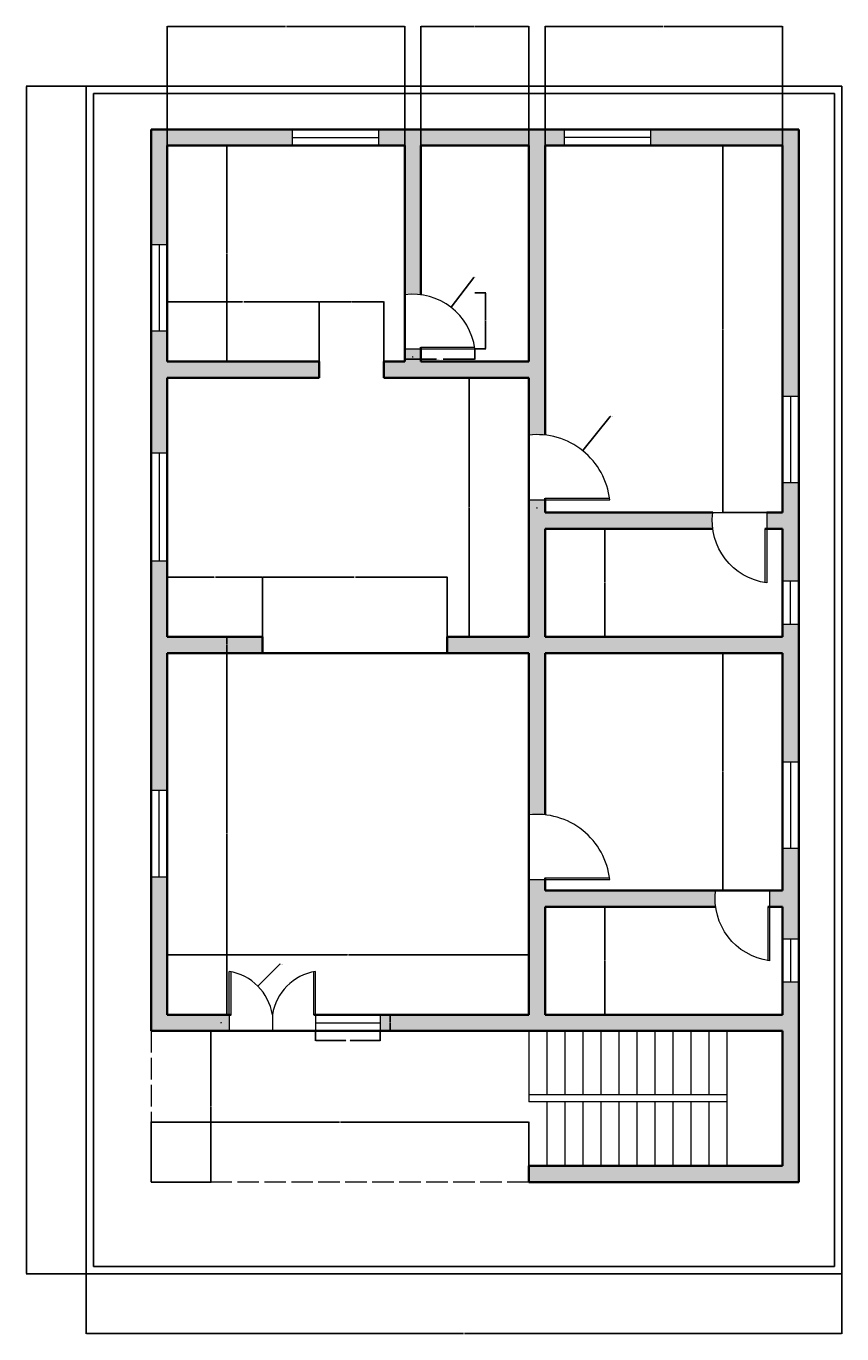
# Model space of a CAD drawing. Units: inches. Extents: x 4948 to 20975, y 6797 to 20508.
# Tile 5 of 5: x 20521 to 20975, y 19252 to 19979. Entities that reach past the tile are written whole.
import ezdxf

# ---------------------------------------------------------------- set-up
doc = ezdxf.new("R2010")
doc.units = ezdxf.units.IN
doc.linetypes.add('ACAD_ISO02W100', pattern=[15, 12, -3])
for name, color, linetype, lineweight in [('A-ANNO-DIMS', 2, 'Continuous', 18), ('A-DOOR', 3, 'Continuous', 18), ('A-FLOR-OVHD', 8, 'ACAD_ISO02W100', 18), ('A-FLOR-STRS', 7, 'Continuous', 18), ('A-GLAZ', 4, 'Continuous', 18), ('A-WALL', 7, 'Continuous', 35), ('C-PROP', 7, 'Continuous', 25)]:
    doc.layers.add(name, color=color, linetype=linetype, lineweight=lineweight)
doc.layers.add('A-WALL-PATT', color=18, linetype='Continuous', lineweight=13, true_color=0x000000)
doc.styles.get("Standard").update_dxf_attribs({"font": 'times.ttf'})
doc.dimstyles.get("Standard").update_dxf_attribs({"dimtxt": 0.18, "dimasz": 0.18, "dimexe": 0.18, "dimexo": 0.0625, "dimgap": 0.09, "dimtad": 0, "dimtih": 1, "dimtoh": 1, "dimdec": 4, "dimzin": 0, "dimdsep": 46, "dimtxsty": 'Standard', "dimcen": 0.09, "dimadec": 0, "dimazin": 0, "dimtfac": 1, "dimtdec": 4, "dimtofl": 0, "dimtmove": 0, "dimatfit": 3, "dimfxl": 1, "dimtolj": 1, "dimtzin": 0, "dimarcsym": 0})

# ---------------------------------------------------------------- blocks, each defined once
blk = doc.blocks.new('DOOR-SINGLE-36IN')
for p, q in [((9, 1), (45, 1)), ((0, 0), (9, 0)), ((9, 0), (45, 0))]:
    blk.add_line(p, q)
blk.add_arc((4.5, -4.5), 40.75, 6.34019, 96.34019)
blk = doc.blocks.new('DOOR-SINGLE-30IN')
for p, q in [((0, 0), (9, 0)), ((9, 1), (39, 1)), ((9, 0), (39, 0))]:
    blk.add_line(p, q)
blk.add_arc((4.5, -4.5), 34.79, 7.43141, 97.43141)
blk = doc.blocks.new('DOOR-DOUBLE-48IN')
for p, q in [((0, 9), (0, 33)), ((1, 9), (1, 33)), ((47, 9), (47, 33)), ((48, 9), (48, 33)), ((0, 9), (0, 0)), ((24, 9), (24, 0)), ((48, 9), (48, 0))]:
    blk.add_line(p, q)
for centre, start, end in [((-4.5, 4.5), 8.97263, 81.02737), ((52.5, 4.5), 98.97263, 171.02737)]:
    blk.add_arc(centre, 28.85, start, end)
blk = doc.blocks.new('WIN-48IN')
for p, q in [((0, 0), (0, 9)), ((48, 0), (48, 9)), ((0, 4.5), (48, 4.5))]:
    blk.add_line(p, q)
blk = doc.blocks.new('WIN-24IN')
for p, q in [((0, 24), (9, 24)), ((4.5, 0), (4.5, 24)), ((0, 0), (9, 0))]:
    blk.add_line(p, q)
blk = doc.blocks.new('WIN-SIDELIGHT-36IN')
for p, q in [((36, 9), (36, 0)), ((0, 4.5), (36, 4.5))]:
    blk.add_line(p, q)
blk = doc.blocks.new('WIN-60IN')
for p, q in [((9, 60), (0, 60)), ((4.5, 60), (4.5, 0)), ((9, 0), (0, 0))]:
    blk.add_line(p, q)
blk = doc.blocks.new('STAIR-RETURN-110IN')
for p, q in [((0, 75), (0, 35.5)), ((10, 75), (10, 39.5)), ((20, 75), (20, 39.5)), ((30, 75), (30, 39.5)), ((40, 75), (40, 39.5)), ((50, 75), (50, 39.5)), ((60, 75), (60, 39.5)), ((70, 75), (70, 39.5)), ((80, 75), (80, 39.5)), ((90, 75), (90, 39.5)), ((100, 75), (100, 39.5)), ((110, 75), (110, 0)), ((110, 39.5), (0, 39.5)), ((110, 35.5), (0, 35.5)), ((10, 35.5), (10, 0)), ((20, 35.5), (20, 0)), ((30, 35.5), (30, 0)), ((40, 35.5), (40, 0)), ((50, 35.5), (50, 0)), ((60, 35.5), (60, 0)), ((70, 35.5), (70, 0)), ((80, 35.5), (80, 0)), ((90, 35.5), (90, 0)), ((100, 35.5), (100, 0))]:
    blk.add_line(p, q)
blk = doc.blocks.new('*D11')
at = {"layer": 'A-ANNO-DIMS', "color": 0, "lineweight": -2, "transparency": 16777216}
for p, q in [((20731.78, 19799.59), (20731.78, 19793.62)), ((20770.78, 19799.59), (20770.78, 19793.62)), ((20731.96, 19793.8), (20749.42, 19793.8)), ((20770.6, 19793.8), (20753.13, 19793.8))]:
    blk.add_line(p, q, dxfattribs=at)
at = {"layer": 'A-ANNO-DIMS', "color": 0, "transparency": 16777216}
for points in [[(20731.96, 19793.83), (20731.96, 19793.77), (20731.78, 19793.8)], [(20770.6, 19793.83), (20770.6, 19793.77), (20770.78, 19793.8)]]:
    blk.add_solid(points, dxfattribs=at)
at = {"layer": 'Defpoints', "color": 0, "transparency": 16777216}
for p in [(20731.78, 19799.65), (20770.78, 19799.65), (20770.78, 19793.8)]:
    blk.add_point(p, dxfattribs=at)
at = {"layer": 'A-ANNO-DIMS', "color": 0, "transparency": 16777216, "insert": (20751.28, 19793.8), "char_height": 0.18, "attachment_point": 5}
blk.add_mtext('\\A1;STORE DOOR SWING 39 TYP.', dxfattribs=at)
blk = doc.blocks.new('*D12')
at = {"layer": 'A-ANNO-DIMS', "color": 0, "lineweight": -2, "transparency": 16777216}
for p, q in [((20770.84, 19830.84), (20776.81, 19830.84)), ((20776.63, 19830.66), (20776.63, 19815.43)), ((20776.63, 19799.83), (20776.63, 19815.06)), ((20770.84, 19799.65), (20776.81, 19799.65))]:
    blk.add_line(p, q, dxfattribs=at)
at = {"layer": 'A-ANNO-DIMS', "color": 0, "transparency": 16777216}
for points in [[(20776.6, 19830.66), (20776.66, 19830.66), (20776.63, 19830.84)], [(20776.6, 19799.83), (20776.66, 19799.83), (20776.63, 19799.65)]]:
    blk.add_solid(points, dxfattribs=at)
at = {"layer": 'Defpoints', "color": 0, "transparency": 16777216}
for p in [(20770.78, 19830.84), (20776.63, 19830.84), (20770.78, 19799.65)]:
    blk.add_point(p, dxfattribs=at)
at = {"layer": 'A-ANNO-DIMS', "color": 0, "transparency": 16777216, "insert": (20776.63, 19815.25), "char_height": 0.18, "attachment_point": 5}
blk.add_mtext('\\A1;31 TYP.', dxfattribs=at)
blk = doc.blocks.new('*D21')
at = {"layer": 'A-ANNO-DIMS', "color": 0, "lineweight": -2, "transparency": 16777216}
for p, q in [((20682.24, 19420.52), (20682.24, 19415)), ((20718.24, 19420.52), (20718.24, 19415)), ((20682.42, 19415.18), (20698.99, 19415.18)), ((20718.06, 19415.18), (20701.49, 19415.18))]:
    blk.add_line(p, q, dxfattribs=at)
at = {"layer": 'A-ANNO-DIMS', "color": 0, "transparency": 16777216}
for points in [[(20682.42, 19415.21), (20682.42, 19415.15), (20682.24, 19415.18)], [(20718.06, 19415.21), (20718.06, 19415.15), (20718.24, 19415.18)]]:
    blk.add_solid(points, dxfattribs=at)
at = {"layer": 'Defpoints', "color": 0, "transparency": 16777216}
for p in [(20682.24, 19420.58), (20718.24, 19420.58), (20718.24, 19415.18)]:
    blk.add_point(p, dxfattribs=at)
at = {"layer": 'A-ANNO-DIMS', "color": 0, "transparency": 16777216, "insert": (20700.24, 19415.18), "char_height": 0.18, "attachment_point": 5}
blk.add_mtext('\\A1;SIDELIGHT 36 TYP.', dxfattribs=at)
blk = doc.blocks.new('*D22')
at = {"layer": 'A-ANNO-DIMS', "color": 0, "lineweight": -2, "transparency": 16777216}
for p, q in [((20718.3, 19429.58), (20723.82, 19429.58)), ((20723.64, 19429.4), (20723.64, 19425.26)), ((20718.3, 19420.58), (20723.82, 19420.58)), ((20723.64, 19420.76), (20723.64, 19424.9))]:
    blk.add_line(p, q, dxfattribs=at)
at = {"layer": 'A-ANNO-DIMS', "color": 0, "transparency": 16777216}
for points in [[(20723.61, 19429.4), (20723.67, 19429.4), (20723.64, 19429.58)], [(20723.61, 19420.76), (20723.67, 19420.76), (20723.64, 19420.58)]]:
    blk.add_solid(points, dxfattribs=at)
at = {"layer": 'Defpoints', "color": 0, "transparency": 16777216}
for p in [(20718.24, 19429.58), (20723.64, 19429.58), (20718.24, 19420.58)]:
    blk.add_point(p, dxfattribs=at)
at = {"layer": 'A-ANNO-DIMS', "color": 0, "transparency": 16777216, "insert": (20723.64, 19425.08), "char_height": 0.18, "attachment_point": 5}
blk.add_mtext('\\A1;9 TYP.', dxfattribs=at)
blk = doc.blocks.new('*D33')
at = {"layer": 'A-ANNO-DIMS', "color": 0, "lineweight": -2, "transparency": 16777216}
for p, q in [((20554.78, 19285.52), (20554.78, 19252.2)), ((20974.78, 19285.52), (20974.78, 19252.2)), ((20554.96, 19252.38), (20764.49, 19252.38)), ((20974.6, 19252.38), (20765.06, 19252.38))]:
    blk.add_line(p, q, dxfattribs=at)
at = {"layer": 'A-ANNO-DIMS', "color": 0, "transparency": 16777216}
for points in [[(20554.96, 19252.41), (20554.96, 19252.35), (20554.78, 19252.38)], [(20974.6, 19252.41), (20974.6, 19252.35), (20974.78, 19252.38)]]:
    blk.add_solid(points, dxfattribs=at)
at = {"layer": 'Defpoints', "color": 0, "transparency": 16777216}
for p in [(20554.78, 19285.58), (20974.78, 19285.58), (20974.78, 19252.38)]:
    blk.add_point(p, dxfattribs=at)
at = {"layer": 'A-ANNO-DIMS', "color": 0, "transparency": 16777216, "insert": (20764.78, 19252.38), "char_height": 0.18, "attachment_point": 5}
blk.add_mtext('\\A1;420', dxfattribs=at)
blk = doc.blocks.new('*D34')
at = {"layer": 'A-ANNO-DIMS', "color": 0, "lineweight": -2, "transparency": 16777216}
for p, q in [((20554.71, 19945.58), (20521.4, 19945.58)), ((20521.58, 19945.4), (20521.58, 19615.76)), ((20521.58, 19285.76), (20521.58, 19615.4)), ((20554.71, 19285.58), (20521.4, 19285.58))]:
    blk.add_line(p, q, dxfattribs=at)
at = {"layer": 'A-ANNO-DIMS', "color": 0, "transparency": 16777216}
for points in [[(20521.55, 19945.4), (20521.61, 19945.4), (20521.58, 19945.58)], [(20521.55, 19285.76), (20521.61, 19285.76), (20521.58, 19285.58)]]:
    blk.add_solid(points, dxfattribs=at)
at = {"layer": 'Defpoints', "color": 0, "transparency": 16777216}
for p in [(20521.58, 19945.58), (20554.78, 19945.58), (20554.78, 19285.58)]:
    blk.add_point(p, dxfattribs=at)
at = {"layer": 'A-ANNO-DIMS', "color": 0, "transparency": 16777216, "insert": (20521.58, 19615.58), "char_height": 0.18, "attachment_point": 5}
blk.add_mtext('\\A1;660', dxfattribs=at)
blk = doc.blocks.new('*D35')
at = {"layer": 'A-ANNO-DIMS', "color": 0, "lineweight": -2, "transparency": 16777216}
for p, q in [((20599.775706, 19912.645372), (20599.775706, 19978.962872)), ((20599.955706, 19978.782872), (20665.507458, 19978.782872)), ((20731.595706, 19978.782872), (20666.043954, 19978.782872)), ((20731.775706, 19912.645372), (20731.775706, 19978.962872))]:
    blk.add_line(p, q, dxfattribs=at)
at = {"layer": 'A-ANNO-DIMS', "color": 0, "transparency": 16777216}
for points in [[(20599.955706, 19978.812872), (20599.955706, 19978.752872), (20599.775706, 19978.782872)], [(20731.595706, 19978.812872), (20731.595706, 19978.752872), (20731.775706, 19978.782872)]]:
    blk.add_solid(points, dxfattribs=at)
at = {"layer": 'Defpoints', "color": 0, "transparency": 16777216}
for p in [(20731.775706, 19978.782872), (20599.775706, 19912.582872), (20731.775706, 19912.582872)]:
    blk.add_point(p, dxfattribs=at)
at = {"layer": 'A-ANNO-DIMS', "color": 0, "transparency": 16777216, "insert": (20665.775706, 19978.782872), "char_height": 0.18, "attachment_point": 5}
blk.add_mtext('\\A1;132', dxfattribs=at)
blk = doc.blocks.new('*D36')
at = {"layer": 'A-ANNO-DIMS', "color": 0, "lineweight": -2, "transparency": 16777216}
for p, q in [((20740.78, 19912.65), (20740.78, 19978.96)), ((20740.96, 19978.78), (20770.56, 19978.78)), ((20800.6, 19978.78), (20770.99, 19978.78)), ((20800.78, 19912.65), (20800.78, 19978.96))]:
    blk.add_line(p, q, dxfattribs=at)
at = {"layer": 'A-ANNO-DIMS', "color": 0, "transparency": 16777216}
for points in [[(20740.96, 19978.81), (20740.96, 19978.75), (20740.78, 19978.78)], [(20800.6, 19978.81), (20800.6, 19978.75), (20800.78, 19978.78)]]:
    blk.add_solid(points, dxfattribs=at)
at = {"layer": 'Defpoints', "color": 0, "transparency": 16777216}
for p in [(20800.78, 19978.78), (20740.78, 19912.58), (20800.78, 19912.58)]:
    blk.add_point(p, dxfattribs=at)
at = {"layer": 'A-ANNO-DIMS', "color": 0, "transparency": 16777216, "insert": (20770.78, 19978.78), "char_height": 0.18, "attachment_point": 5}
blk.add_mtext('\\A1;60', dxfattribs=at)
blk = doc.blocks.new('*D37')
at = {"layer": 'A-ANNO-DIMS', "color": 0, "lineweight": -2, "transparency": 16777216}
for p, q in [((20809.775706, 19912.645372), (20809.775706, 19978.962872)), ((20809.955706, 19978.782872), (20875.507458, 19978.782872)), ((20941.595706, 19978.782872), (20876.043954, 19978.782872)), ((20941.775706, 19912.645372), (20941.775706, 19978.962872))]:
    blk.add_line(p, q, dxfattribs=at)
at = {"layer": 'A-ANNO-DIMS', "color": 0, "transparency": 16777216}
for points in [[(20809.955706, 19978.812872), (20809.955706, 19978.752872), (20809.775706, 19978.782872)], [(20941.595706, 19978.812872), (20941.595706, 19978.752872), (20941.775706, 19978.782872)]]:
    blk.add_solid(points, dxfattribs=at)
at = {"layer": 'Defpoints', "color": 0, "transparency": 16777216}
for p in [(20941.775706, 19978.782872), (20809.775706, 19912.582872), (20941.775706, 19912.582872)]:
    blk.add_point(p, dxfattribs=at)
at = {"layer": 'A-ANNO-DIMS', "color": 0, "transparency": 16777216, "insert": (20875.775706, 19978.782872), "char_height": 0.18, "attachment_point": 5}
blk.add_mtext('\\A1;132', dxfattribs=at)
blk = doc.blocks.new('*D38')
at = {"layer": 'A-ANNO-DIMS', "color": 0, "lineweight": -2, "transparency": 16777216}
for p, q in [((20599.84, 19912.58), (20633.16, 19912.58)), ((20632.98, 19912.4), (20632.98, 19852.76)), ((20632.98, 19792.76), (20632.98, 19852.4)), ((20599.84, 19792.58), (20633.16, 19792.58))]:
    blk.add_line(p, q, dxfattribs=at)
at = {"layer": 'A-ANNO-DIMS', "color": 0, "transparency": 16777216}
for points in [[(20632.95, 19912.4), (20633.01, 19912.4), (20632.98, 19912.58)], [(20632.95, 19792.76), (20633.01, 19792.76), (20632.98, 19792.58)]]:
    blk.add_solid(points, dxfattribs=at)
at = {"layer": 'Defpoints', "color": 0, "transparency": 16777216}
for p in [(20599.78, 19912.58), (20599.78, 19792.58), (20632.98, 19792.58)]:
    blk.add_point(p, dxfattribs=at)
at = {"layer": 'A-ANNO-DIMS', "color": 0, "transparency": 16777216, "insert": (20632.98, 19852.58), "char_height": 0.18, "attachment_point": 5}
blk.add_mtext('\\A1;120', dxfattribs=at)
blk = doc.blocks.new('*D39')
at = {"layer": 'A-ANNO-DIMS', "color": 0, "lineweight": -2, "transparency": 16777216}
for p, q in [((20800.713206, 19783.582872), (20767.395706, 19783.582872)), ((20767.575706, 19783.402872), (20767.575706, 19711.762872)), ((20767.575706, 19639.762872), (20767.575706, 19711.402872)), ((20800.713206, 19639.582872), (20767.395706, 19639.582872))]:
    blk.add_line(p, q, dxfattribs=at)
at = {"layer": 'A-ANNO-DIMS', "color": 0, "transparency": 16777216}
for points in [[(20767.545706, 19783.402872), (20767.605706, 19783.402872), (20767.575706, 19783.582872)], [(20767.545706, 19639.762872), (20767.605706, 19639.762872), (20767.575706, 19639.582872)]]:
    blk.add_solid(points, dxfattribs=at)
at = {"layer": 'Defpoints', "color": 0, "transparency": 16777216}
for p in [(20767.575706, 19783.582872), (20800.775706, 19783.582872), (20800.775706, 19639.582872)]:
    blk.add_point(p, dxfattribs=at)
at = {"layer": 'A-ANNO-DIMS', "color": 0, "transparency": 16777216, "insert": (20767.575706, 19711.582872), "char_height": 0.18, "attachment_point": 5}
blk.add_mtext('\\A1;144', dxfattribs=at)
blk = doc.blocks.new('*D40')
at = {"layer": 'A-ANNO-DIMS', "color": 0, "lineweight": -2, "transparency": 16777216}
for p, q in [((20599.84, 19630.58), (20633.16, 19630.58)), ((20632.98, 19630.4), (20632.98, 19530.26)), ((20632.98, 19429.76), (20632.98, 19529.9)), ((20599.84, 19429.58), (20633.16, 19429.58))]:
    blk.add_line(p, q, dxfattribs=at)
at = {"layer": 'A-ANNO-DIMS', "color": 0, "transparency": 16777216}
for points in [[(20632.95, 19630.4), (20633.01, 19630.4), (20632.98, 19630.58)], [(20632.95, 19429.76), (20633.01, 19429.76), (20632.98, 19429.58)]]:
    blk.add_solid(points, dxfattribs=at)
at = {"layer": 'Defpoints', "color": 0, "transparency": 16777216}
for p in [(20599.78, 19630.58), (20599.78, 19429.58), (20632.98, 19429.58)]:
    blk.add_point(p, dxfattribs=at)
at = {"layer": 'A-ANNO-DIMS', "color": 0, "transparency": 16777216, "insert": (20632.98, 19530.08), "char_height": 0.18, "attachment_point": 5}
blk.add_mtext('\\A1;201', dxfattribs=at)
blk = doc.blocks.new('*D41')
at = {"layer": 'A-ANNO-DIMS', "color": 0, "lineweight": -2, "transparency": 16777216}
for p, q in [((20941.71, 19912.58), (20908.4, 19912.58)), ((20908.58, 19912.4), (20908.58, 19810.76)), ((20908.58, 19708.76), (20908.58, 19810.4)), ((20941.71, 19708.58), (20908.4, 19708.58))]:
    blk.add_line(p, q, dxfattribs=at)
at = {"layer": 'A-ANNO-DIMS', "color": 0, "transparency": 16777216}
for points in [[(20908.55, 19912.4), (20908.61, 19912.4), (20908.58, 19912.58)], [(20908.55, 19708.76), (20908.61, 19708.76), (20908.58, 19708.58)]]:
    blk.add_solid(points, dxfattribs=at)
at = {"layer": 'Defpoints', "color": 0, "transparency": 16777216}
for p in [(20908.58, 19912.58), (20941.78, 19912.58), (20941.78, 19708.58)]:
    blk.add_point(p, dxfattribs=at)
at = {"layer": 'A-ANNO-DIMS', "color": 0, "transparency": 16777216, "insert": (20908.58, 19810.58), "char_height": 0.18, "attachment_point": 5}
blk.add_mtext('\\A1;204', dxfattribs=at)
blk = doc.blocks.new('*D42')
at = {"layer": 'A-ANNO-DIMS', "color": 0, "lineweight": -2, "transparency": 16777216}
for p, q in [((20809.84, 19699.58), (20843.16, 19699.58)), ((20842.98, 19699.4), (20842.98, 19669.76)), ((20842.98, 19639.76), (20842.98, 19669.4)), ((20809.84, 19639.58), (20843.16, 19639.58))]:
    blk.add_line(p, q, dxfattribs=at)
at = {"layer": 'A-ANNO-DIMS', "color": 0, "transparency": 16777216}
for points in [[(20842.95, 19699.4), (20843.01, 19699.4), (20842.98, 19699.58)], [(20842.95, 19639.76), (20843.01, 19639.76), (20842.98, 19639.58)]]:
    blk.add_solid(points, dxfattribs=at)
at = {"layer": 'Defpoints', "color": 0, "transparency": 16777216}
for p in [(20809.78, 19699.58), (20809.78, 19639.58), (20842.98, 19639.58)]:
    blk.add_point(p, dxfattribs=at)
at = {"layer": 'A-ANNO-DIMS', "color": 0, "transparency": 16777216, "insert": (20842.98, 19669.58), "char_height": 0.18, "attachment_point": 5}
blk.add_mtext('\\A1;60', dxfattribs=at)
blk = doc.blocks.new('*D43')
at = {"layer": 'A-ANNO-DIMS', "color": 0, "lineweight": -2, "transparency": 16777216}
for p, q in [((20941.71, 19630.58), (20908.4, 19630.58)), ((20908.58, 19630.4), (20908.58, 19564.76)), ((20908.58, 19498.76), (20908.58, 19564.4)), ((20941.71, 19498.58), (20908.4, 19498.58))]:
    blk.add_line(p, q, dxfattribs=at)
at = {"layer": 'A-ANNO-DIMS', "color": 0, "transparency": 16777216}
for points in [[(20908.55, 19630.4), (20908.61, 19630.4), (20908.58, 19630.58)], [(20908.55, 19498.76), (20908.61, 19498.76), (20908.58, 19498.58)]]:
    blk.add_solid(points, dxfattribs=at)
at = {"layer": 'Defpoints', "color": 0, "transparency": 16777216}
for p in [(20908.58, 19630.58), (20941.78, 19630.58), (20941.78, 19498.58)]:
    blk.add_point(p, dxfattribs=at)
at = {"layer": 'A-ANNO-DIMS', "color": 0, "transparency": 16777216, "insert": (20908.58, 19564.58), "char_height": 0.18, "attachment_point": 5}
blk.add_mtext('\\A1;132', dxfattribs=at)
blk = doc.blocks.new('*D44')
at = {"layer": 'A-ANNO-DIMS', "color": 0, "lineweight": -2, "transparency": 16777216}
for p, q in [((20809.84, 19489.58), (20843.16, 19489.58)), ((20842.98, 19489.4), (20842.98, 19459.76)), ((20842.98, 19429.76), (20842.98, 19459.4)), ((20809.84, 19429.58), (20843.16, 19429.58))]:
    blk.add_line(p, q, dxfattribs=at)
at = {"layer": 'A-ANNO-DIMS', "color": 0, "transparency": 16777216}
for points in [[(20842.95, 19489.4), (20843.01, 19489.4), (20842.98, 19489.58)], [(20842.95, 19429.76), (20843.01, 19429.76), (20842.98, 19429.58)]]:
    blk.add_solid(points, dxfattribs=at)
at = {"layer": 'Defpoints', "color": 0, "transparency": 16777216}
for p in [(20809.78, 19489.58), (20809.78, 19429.58), (20842.98, 19429.58)]:
    blk.add_point(p, dxfattribs=at)
at = {"layer": 'A-ANNO-DIMS', "color": 0, "transparency": 16777216, "insert": (20842.98, 19459.58), "char_height": 0.18, "attachment_point": 5}
blk.add_mtext('\\A1;60', dxfattribs=at)
blk = doc.blocks.new('*D45')
at = {"layer": 'A-ANNO-DIMS', "color": 0, "lineweight": -2, "transparency": 16777216}
for p, q in [((20599.78, 19429.65), (20599.78, 19462.96)), ((20599.96, 19462.78), (20700.01, 19462.78)), ((20800.6, 19462.78), (20700.55, 19462.78)), ((20800.78, 19429.65), (20800.78, 19462.96))]:
    blk.add_line(p, q, dxfattribs=at)
at = {"layer": 'A-ANNO-DIMS', "color": 0, "transparency": 16777216}
for points in [[(20599.96, 19462.81), (20599.96, 19462.75), (20599.78, 19462.78)], [(20800.6, 19462.81), (20800.6, 19462.75), (20800.78, 19462.78)]]:
    blk.add_solid(points, dxfattribs=at)
at = {"layer": 'Defpoints', "color": 0, "transparency": 16777216}
for p in [(20800.78, 19462.78), (20599.78, 19429.58), (20800.78, 19429.58)]:
    blk.add_point(p, dxfattribs=at)
at = {"layer": 'A-ANNO-DIMS', "color": 0, "transparency": 16777216, "insert": (20700.28, 19462.78), "char_height": 0.18, "attachment_point": 5}
blk.add_mtext('\\A1;201', dxfattribs=at)
blk = doc.blocks.new('*D46')
at = {"layer": 'A-ANNO-DIMS', "color": 0, "lineweight": -2, "transparency": 16777216}
for p, q in [((20590.78, 19336.65), (20590.78, 19369.96)), ((20590.96, 19369.78), (20695.49, 19369.78)), ((20800.6, 19369.78), (20696.06, 19369.78)), ((20800.78, 19336.65), (20800.78, 19369.96))]:
    blk.add_line(p, q, dxfattribs=at)
at = {"layer": 'A-ANNO-DIMS', "color": 0, "transparency": 16777216}
for points in [[(20590.96, 19369.81), (20590.96, 19369.75), (20590.78, 19369.78)], [(20800.6, 19369.81), (20800.6, 19369.75), (20800.78, 19369.78)]]:
    blk.add_solid(points, dxfattribs=at)
at = {"layer": 'Defpoints', "color": 0, "transparency": 16777216}
for p in [(20800.78, 19369.78), (20590.78, 19336.58), (20800.78, 19336.58)]:
    blk.add_point(p, dxfattribs=at)
at = {"layer": 'A-ANNO-DIMS', "color": 0, "transparency": 16777216, "insert": (20695.78, 19369.78), "char_height": 0.18, "attachment_point": 5}
blk.add_mtext('\\A1;210', dxfattribs=at)
blk = doc.blocks.new('*D47')
at = {"layer": 'A-ANNO-DIMS', "color": 0, "lineweight": -2, "transparency": 16777216}
for p, q in [((20590.84, 19420.58), (20624.16, 19420.58)), ((20623.98, 19420.4), (20623.98, 19378.76)), ((20623.98, 19336.76), (20623.98, 19378.4)), ((20590.84, 19336.58), (20624.16, 19336.58))]:
    blk.add_line(p, q, dxfattribs=at)
at = {"layer": 'A-ANNO-DIMS', "color": 0, "transparency": 16777216}
for points in [[(20623.95, 19420.4), (20624.01, 19420.4), (20623.98, 19420.58)], [(20623.95, 19336.76), (20624.01, 19336.76), (20623.98, 19336.58)]]:
    blk.add_solid(points, dxfattribs=at)
at = {"layer": 'Defpoints', "color": 0, "transparency": 16777216}
for p in [(20590.78, 19420.58), (20590.78, 19336.58), (20623.98, 19336.58)]:
    blk.add_point(p, dxfattribs=at)
at = {"layer": 'A-ANNO-DIMS', "color": 0, "transparency": 16777216, "insert": (20623.98, 19378.58), "char_height": 0.18, "attachment_point": 5}
blk.add_mtext('\\A1;84', dxfattribs=at)
blk = doc.blocks.new('*D48')
at = {"layer": 'A-ANNO-DIMS', "color": 0, "lineweight": -2, "transparency": 16777216}
for p, q in [((20599.78, 19792.65), (20599.78, 19825.96)), ((20599.96, 19825.78), (20641.63, 19825.78)), ((20684.06, 19825.78), (20642.38, 19825.78)), ((20684.24, 19792.65), (20684.24, 19825.96))]:
    blk.add_line(p, q, dxfattribs=at)
at = {"layer": 'A-ANNO-DIMS', "color": 0, "transparency": 16777216}
for points in [[(20599.96, 19825.81), (20599.96, 19825.75), (20599.78, 19825.78)], [(20684.06, 19825.81), (20684.06, 19825.75), (20684.24, 19825.78)]]:
    blk.add_solid(points, dxfattribs=at)
at = {"layer": 'Defpoints', "color": 0, "transparency": 16777216}
for p in [(20684.24, 19825.78), (20599.78, 19792.58), (20684.24, 19792.58)]:
    blk.add_point(p, dxfattribs=at)
at = {"layer": 'A-ANNO-DIMS', "color": 0, "transparency": 16777216, "insert": (20642.01, 19825.78), "char_height": 0.18, "attachment_point": 5}
blk.add_mtext('\\A1;84.47', dxfattribs=at)
blk = doc.blocks.new('*D49')
at = {"layer": 'A-ANNO-DIMS', "color": 0, "lineweight": -2, "transparency": 16777216}
for p, q in [((20684.24, 19792.65), (20684.24, 19825.96)), ((20684.42, 19825.78), (20702.03, 19825.78)), ((20720.06, 19825.78), (20702.46, 19825.78)), ((20720.24, 19792.65), (20720.24, 19825.96))]:
    blk.add_line(p, q, dxfattribs=at)
at = {"layer": 'A-ANNO-DIMS', "color": 0, "transparency": 16777216}
for points in [[(20684.42, 19825.81), (20684.42, 19825.75), (20684.24, 19825.78)], [(20720.06, 19825.81), (20720.06, 19825.75), (20720.24, 19825.78)]]:
    blk.add_solid(points, dxfattribs=at)
at = {"layer": 'Defpoints', "color": 0, "transparency": 16777216}
for p in [(20720.24, 19825.78), (20684.24, 19792.58), (20720.24, 19792.58)]:
    blk.add_point(p, dxfattribs=at)
at = {"layer": 'A-ANNO-DIMS', "color": 0, "transparency": 16777216, "insert": (20702.24, 19825.78), "char_height": 0.18, "attachment_point": 5}
blk.add_mtext('\\A1;36', dxfattribs=at)
blk = doc.blocks.new('*D50')
at = {"layer": 'A-ANNO-DIMS', "color": 0, "lineweight": -2, "transparency": 16777216}
for p, q in [((20599.78, 19639.65), (20599.78, 19672.96)), ((20599.96, 19672.78), (20625.88, 19672.78)), ((20652.56, 19672.78), (20626.64, 19672.78)), ((20652.74, 19639.65), (20652.74, 19672.96))]:
    blk.add_line(p, q, dxfattribs=at)
at = {"layer": 'A-ANNO-DIMS', "color": 0, "transparency": 16777216}
for points in [[(20599.96, 19672.81), (20599.96, 19672.75), (20599.78, 19672.78)], [(20652.56, 19672.81), (20652.56, 19672.75), (20652.74, 19672.78)]]:
    blk.add_solid(points, dxfattribs=at)
at = {"layer": 'Defpoints', "color": 0, "transparency": 16777216}
for p in [(20652.74, 19672.78), (20599.78, 19639.58), (20652.74, 19639.58)]:
    blk.add_point(p, dxfattribs=at)
at = {"layer": 'A-ANNO-DIMS', "color": 0, "transparency": 16777216, "insert": (20626.26, 19672.78), "char_height": 0.18, "attachment_point": 5}
blk.add_mtext('\\A1;52.97', dxfattribs=at)
blk = doc.blocks.new('*D51')
at = {"layer": 'A-ANNO-DIMS', "color": 0, "lineweight": -2, "transparency": 16777216}
for p, q in [((20652.74, 19639.65), (20652.74, 19672.96)), ((20652.92, 19672.78), (20703.63, 19672.78)), ((20755.2, 19672.78), (20704.5, 19672.78)), ((20755.38, 19639.65), (20755.38, 19672.96))]:
    blk.add_line(p, q, dxfattribs=at)
at = {"layer": 'A-ANNO-DIMS', "color": 0, "transparency": 16777216}
for points in [[(20652.92, 19672.81), (20652.92, 19672.75), (20652.74, 19672.78)], [(20755.2, 19672.81), (20755.2, 19672.75), (20755.38, 19672.78)]]:
    blk.add_solid(points, dxfattribs=at)
at = {"layer": 'Defpoints', "color": 0, "transparency": 16777216}
for p in [(20755.38, 19672.78), (20652.74, 19639.58), (20755.38, 19639.58)]:
    blk.add_point(p, dxfattribs=at)
at = {"layer": 'A-ANNO-DIMS', "color": 0, "transparency": 16777216, "insert": (20704.06, 19672.78), "char_height": 0.18, "attachment_point": 5}
blk.add_mtext('\\A1;102.64', dxfattribs=at)
blk = doc.blocks.new('*D52')
at = {"layer": 'A-ANNO-DIMS', "color": 0, "lineweight": -2, "transparency": 16777216}
for p, q in [((20599.84, 19639.58), (20633.16, 19639.58)), ((20632.98, 19639.4), (20632.98, 19635.26)), ((20599.84, 19630.58), (20633.16, 19630.58)), ((20632.98, 19630.76), (20632.98, 19634.9))]:
    blk.add_line(p, q, dxfattribs=at)
at = {"layer": 'A-ANNO-DIMS', "color": 0, "transparency": 16777216}
for points in [[(20632.95, 19639.4), (20633.01, 19639.4), (20632.98, 19639.58)], [(20632.95, 19630.76), (20633.01, 19630.76), (20632.98, 19630.58)]]:
    blk.add_solid(points, dxfattribs=at)
at = {"layer": 'Defpoints', "color": 0, "transparency": 16777216}
for p in [(20599.78, 19639.58), (20599.78, 19630.58), (20632.98, 19630.58)]:
    blk.add_point(p, dxfattribs=at)
at = {"layer": 'A-ANNO-DIMS', "color": 0, "transparency": 16777216, "insert": (20632.98, 19635.08), "char_height": 0.18, "attachment_point": 5}
blk.add_mtext('\\A1;9', dxfattribs=at)
blk = doc.blocks.new('*D90')
at = {"layer": 'A-ANNO-DIMS', "color": 0, "lineweight": -2, "transparency": 16777216}
for p, q in [((20846.01, 19762.1), (20830.84, 19743.15)), ((20846.19, 19762.1), (20846.01, 19762.1)), ((20805.19, 19711.19), (20805.37, 19711.19)), ((20805.28, 19711.1), (20805.28, 19711.28))]:
    blk.add_line(p, q, dxfattribs=at)
at = {"layer": 'A-ANNO-DIMS', "color": 0, "transparency": 16777216}
blk.add_solid([(20830.82, 19743.17), (20830.87, 19743.13), (20830.73, 19743.01)], dxfattribs=at)
at = {"layer": 'Defpoints', "color": 0, "transparency": 16777216}
for p in [(20830.73, 19743.01), (20805.28, 19711.19)]:
    blk.add_point(p, dxfattribs=at)
at = {"layer": 'A-ANNO-DIMS', "color": 0, "transparency": 16777216, "insert": (20846.85, 19762.1), "char_height": 0.18, "attachment_point": 5}
blk.add_mtext('\\A1;2X R40.75', dxfattribs=at)
blk = doc.blocks.new('*D91')
at = {"layer": 'A-ANNO-DIMS', "color": 0, "lineweight": -2, "transparency": 16777216}
for p, q in [((20770.22, 19839.27), (20757.6, 19822.87)), ((20770.4, 19839.27), (20770.22, 19839.27)), ((20736.19, 19795.15), (20736.37, 19795.15)), ((20736.28, 19795.06), (20736.28, 19795.24))]:
    blk.add_line(p, q, dxfattribs=at)
at = {"layer": 'A-ANNO-DIMS', "color": 0, "transparency": 16777216}
blk.add_solid([(20757.58, 19822.89), (20757.62, 19822.85), (20757.49, 19822.73)], dxfattribs=at)
at = {"layer": 'Defpoints', "color": 0, "transparency": 16777216}
for p in [(20757.49, 19822.73), (20736.28, 19795.15)]:
    blk.add_point(p, dxfattribs=at)
at = {"layer": 'A-ANNO-DIMS', "color": 0, "transparency": 16777216, "insert": (20770.87, 19839.27), "char_height": 0.18, "attachment_point": 5}
blk.add_mtext('\\A1;R34.79', dxfattribs=at)
blk = doc.blocks.new('*D92')
at = {"layer": 'A-ANNO-DIMS', "color": 0, "lineweight": -2, "transparency": 16777216}
for p, q in [((20662.38, 19457.73), (20650.27, 19445.61)), ((20662.56, 19457.73), (20662.38, 19457.73)), ((20629.65, 19425.08), (20629.83, 19425.08)), ((20629.74, 19424.99), (20629.74, 19425.17))]:
    blk.add_line(p, q, dxfattribs=at)
at = {"layer": 'A-ANNO-DIMS', "color": 0, "transparency": 16777216}
blk.add_solid([(20650.25, 19445.63), (20650.29, 19445.59), (20650.14, 19445.48)], dxfattribs=at)
at = {"layer": 'Defpoints', "color": 0, "transparency": 16777216}
for p in [(20650.14, 19445.48), (20629.74, 19425.08)]:
    blk.add_point(p, dxfattribs=at)
at = {"layer": 'A-ANNO-DIMS', "color": 0, "transparency": 16777216, "insert": (20663.29, 19457.73), "char_height": 0.18, "attachment_point": 5}
blk.add_mtext('\\A1;2X R28.853', dxfattribs=at)

msp = doc.modelspace()

# ---------------------------------------------------------------- hatches: boundary and pattern name
at = {"layer": 'A-WALL-PATT'}
h = msp.add_hatch(color=256, dxfattribs=at)
h.dxf.hatch_style = 1
h.paths.add_polyline_path([(20669.3971, 19921.5829), (20590.7757, 19921.5829), (20590.7757, 19857.674), (20599.7757, 19857.674), (20599.7757, 19912.5829), (20669.3971, 19912.5829)])
h.paths.add_polyline_path([(20820.4356, 19921.5829), (20717.3971, 19921.5829), (20717.3971, 19912.5829), (20731.7757, 19912.5829), (20731.7757, 19829.6483, -0.06494234), (20740.7757, 19829.6483), (20740.7757, 19912.5829), (20800.7757, 19912.5829), (20800.7757, 19792.5829), (20740.7757, 19792.5829), (20740.7757, 19799.6483), (20731.7757, 19799.6483), (20731.7757, 19792.5829), (20720.244, 19792.5829), (20720.244, 19783.5829), (20800.7757, 19783.5829), (20800.7757, 19751.6915, -0.05538514), (20809.7757, 19751.6915), (20809.7757, 19783.5829), (20809.7757, 19912.5829), (20820.4356, 19912.5829)])
h.paths.add_polyline_path([(20950.7757, 19921.5829), (20868.4356, 19921.5829), (20868.4356, 19912.5829), (20941.7757, 19912.5829), (20941.7757, 19773.2876), (20950.7757, 19773.2876)])
h.paths.add_polyline_path([(20599.7757, 19783.5829), (20684.244, 19783.5829), (20684.244, 19792.5829), (20599.7757, 19792.5829), (20599.7757, 19809.674), (20590.7757, 19809.674), (20590.7757, 19741.5829), (20599.7757, 19741.5829)])
h.paths.add_polyline_path([(20950.7757, 19646.681), (20941.7757, 19646.681), (20941.7757, 19639.5829), (20809.7757, 19639.5829), (20809.7757, 19699.5829), (20903.0134, 19699.5829, -0.06494234), (20903.0134, 19708.5829), (20809.7757, 19708.5829), (20809.7757, 19715.6915), (20800.7757, 19715.6915), (20800.7757, 19699.5829), (20800.7757, 19639.5829), (20755.3794, 19639.5829), (20755.3794, 19630.5829), (20800.7757, 19630.5829), (20800.7757, 19540.6607, -0.05538514), (20809.7757, 19540.6607), (20809.7757, 19630.5829), (20941.7757, 19630.5829), (20941.7757, 19570.0343), (20950.7757, 19570.0343)])
h.paths.add_polyline_path([(20950.7757, 19725.2876), (20941.7757, 19725.2876), (20941.7757, 19708.5829), (20933.0134, 19708.5829), (20933.0134, 19699.5829), (20941.7757, 19699.5829), (20941.7757, 19670.681), (20950.7757, 19670.681)])
h.paths.add_polyline_path([(20950.7757, 19522.0343), (20941.7757, 19522.0343), (20941.7757, 19498.5829), (20934.6125, 19498.5829), (20934.6125, 19489.5829), (20941.7757, 19489.5829), (20941.7757, 19471.5829), (20950.7757, 19471.5829)])
h.paths.add_polyline_path([(20950.7757, 19447.5829), (20941.7757, 19447.5829), (20941.7757, 19429.5829), (20809.7757, 19429.5829), (20809.7757, 19489.5829), (20904.6125, 19489.5829, -0.06494234), (20904.6125, 19498.5829), (20809.7757, 19498.5829), (20809.7757, 19504.6607), (20800.7757, 19504.6607), (20800.7757, 19429.5829), (20718.2384, 19429.5829), (20718.2384, 19420.5829), (20800.7757, 19420.5829), (20809.7757, 19420.5829), (20941.7757, 19420.5829), (20941.7757, 19345.5829), (20800.7757, 19345.5829), (20800.7757, 19336.5829), (20950.7757, 19336.5829)])
h.paths.add_polyline_path([(20634.2384, 19429.5829), (20599.7757, 19429.5829), (20599.7757, 19506.0829), (20590.7757, 19506.0829), (20590.7757, 19420.5829), (20599.7757, 19420.5829), (20634.2384, 19420.5829)])
h.paths.add_polyline_path([(20599.7757, 19630.5829), (20652.742, 19630.5829), (20652.742, 19639.5829), (20599.7757, 19639.5829), (20599.7757, 19681.5829), (20590.7757, 19681.5829), (20590.7757, 19554.0829), (20599.7757, 19554.0829)])

# ---------------------------------------------------------------- linework, layer by layer
at = {"layer": 'A-DOOR'}
msp.add_line((20903.0134, 19708.5829), (20933.0134, 19708.5829), dxfattribs=at)
at = {"layer": 'A-FLOR-OVHD'}
for p in [(20590.7757, 19420.5829), (20800.7757, 19336.5829)]:
    msp.add_line(p, (20590.7757, 19336.5829), dxfattribs=at)
at = {"layer": 'A-WALL'}
for p, q in [((20590.7757, 19921.5829), (20950.7757, 19921.5829)), ((20590.7757, 19420.5829), (20590.7757, 19921.5829)), ((20950.7757, 19921.5829), (20950.7757, 19336.5829)), ((20599.7757, 19912.5829), (20731.7757, 19912.5829)), ((20599.7757, 19792.5829), (20599.7757, 19912.5829)), ((20731.7757, 19792.5829), (20731.7757, 19912.5829)), ((20740.7757, 19912.5829), (20800.7757, 19912.5829)), ((20740.7757, 19829.6483), (20740.7757, 19912.5829)), ((20800.7757, 19792.5829), (20800.7757, 19912.5829)), ((20809.7757, 19912.5829), (20941.7757, 19912.5829)), ((20809.7757, 19783.5829), (20809.7757, 19912.5829)), ((20941.7757, 19912.5829), (20941.7757, 19708.5829)), ((20740.7757, 19792.5829), (20740.7757, 19800.6483)), ((20599.7757, 19792.5829), (20684.244, 19792.5829)), ((20684.244, 19792.5829), (20684.244, 19783.5829)), ((20720.244, 19792.5829), (20731.7757, 19792.5829)), ((20720.244, 19792.5829), (20720.244, 19783.5829)), ((20740.7757, 19792.5829), (20800.7757, 19792.5829)), ((20599.7757, 19783.5829), (20684.244, 19783.5829)), ((20599.7757, 19639.5829), (20599.7757, 19783.5829)), ((20720.244, 19783.5829), (20800.7757, 19783.5829)), ((20800.7757, 19783.5829), (20800.7757, 19699.5829)), ((20809.7757, 19783.5829), (20809.7757, 19751.6915)), ((20809.7757, 19716.6915), (20809.7757, 19708.5829)), ((20809.7757, 19708.5829), (20903.0134, 19708.5829)), ((20933.0134, 19708.5829), (20941.7757, 19708.5829)), ((20800.7757, 19699.5829), (20800.7757, 19639.5829)), ((20809.7757, 19699.5829), (20903.0134, 19699.5829)), ((20809.7757, 19699.5829), (20809.7757, 19639.5829)), ((20932.0134, 19699.5829), (20941.7757, 19699.5829)), ((20941.7757, 19699.5829), (20941.7757, 19639.5829)), ((20599.7757, 19639.5829), (20652.742, 19639.5829)), ((20652.742, 19630.5829), (20652.742, 19639.5829)), ((20755.3794, 19639.5829), (20800.7757, 19639.5829)), ((20755.3794, 19630.5829), (20755.3794, 19639.5829)), ((20809.7757, 19639.5829), (20941.7757, 19639.5829)), ((20599.7757, 19630.5829), (20652.742, 19630.5829)), ((20599.7757, 19429.5829), (20599.7757, 19630.5829)), ((20652.742, 19630.5829), (20755.3794, 19630.5829)), ((20755.3794, 19630.5829), (20800.7757, 19630.5829)), ((20800.7757, 19630.5829), (20800.7757, 19429.5829)), ((20809.7757, 19630.5829), (20809.7757, 19540.6607)), ((20809.7757, 19630.5829), (20941.7757, 19630.5829)), ((20941.7757, 19630.5829), (20941.7757, 19498.5829)), ((20809.7757, 19505.6607), (20809.7757, 19498.5829)), ((20809.7757, 19498.5829), (20941.7757, 19498.5829)), ((20809.7757, 19489.5829), (20809.7757, 19429.5829)), ((20809.7757, 19489.5829), (20904.6125, 19489.5829)), ((20933.6125, 19489.5829), (20941.7757, 19489.5829)), ((20941.7757, 19489.5829), (20941.7757, 19429.5829)), ((20599.7757, 19429.5829), (20635.2384, 19429.5829)), ((20681.2384, 19429.5829), (20800.7757, 19429.5829)), ((20809.7757, 19429.5829), (20941.7757, 19429.5829)), ((20599.7757, 19420.5829), (20590.7757, 19420.5829)), ((20599.7757, 19420.5829), (20800.7757, 19420.5829)), ((20800.7757, 19420.5829), (20809.7757, 19420.5829)), ((20809.7757, 19420.5829), (20941.7757, 19420.5829)), ((20941.7757, 19420.5829), (20941.7757, 19345.5829)), ((20941.7757, 19345.5829), (20800.7757, 19345.5829)), ((20800.7757, 19345.5829), (20800.7757, 19336.5829)), ((20950.7757, 19336.5829), (20800.7757, 19336.5829))]:
    msp.add_line(p, q, dxfattribs=at)
at = {"layer": 'C-PROP'}
for p, q in [((20554.7757, 19945.5829), (20974.7757, 19945.5829)), ((20554.7757, 19285.5829), (20554.7757, 19945.5829)), ((20974.7757, 19945.5829), (20974.7757, 19285.5829)), ((20558.7757, 19941.5829), (20970.7757, 19941.5829)), ((20558.7757, 19289.5829), (20558.7757, 19941.5829)), ((20970.7757, 19941.5829), (20970.7757, 19289.5829)), ((20970.7757, 19289.5829), (20558.7757, 19289.5829)), ((20974.7757, 19285.5829), (20554.7757, 19285.5829))]:
    msp.add_line(p, q, dxfattribs=at)

# ---------------------------------------------------------------- block references
at = {"layer": 'A-DOOR'}
for name, p in [('DOOR-SINGLE-30IN', (20731.7758, 19799.6478)), ('DOOR-SINGLE-36IN', (20800.7758, 19715.6918)), ('DOOR-SINGLE-36IN', (20800.7758, 19504.6611)), ('DOOR-DOUBLE-48IN', (20634.2388, 19420.5828))]:
    msp.add_blockref(name, p, dxfattribs=at)
at = {"layer": 'A-DOOR', "extrusion": (0, 0, -1), "zscale": -1, "rotation": 270.0000000000202}
for p in [(-20933.0138, 19708.5828), (-20934.613, 19498.5828)]:
    msp.add_blockref('DOOR-SINGLE-30IN', p, dxfattribs=at)
at = {"layer": 'A-FLOR-STRS'}
msp.add_blockref('STAIR-RETURN-110IN', (20800.7758, 19345.5828), dxfattribs=at)
at = {"layer": 'A-GLAZ'}
for name, p in [('WIN-48IN', (20669.3968, 19912.5828)), ('WIN-60IN', (20590.7758, 19681.5828)), ('WIN-24IN', (20941.7758, 19646.6808)), ('WIN-SIDELIGHT-36IN', (20682.2388, 19420.5828))]:
    msp.add_blockref(name, p, dxfattribs=at)
for name, p, rotation in [('WIN-48IN', (20868.436, 19921.5829), 180), ('WIN-48IN', (20590.7757, 19857.6744), 269.9999999999846), ('WIN-48IN', (20941.7757, 19773.288), 269.9999999999846), ('WIN-48IN', (20941.7757, 19570.0347), 270.0000000000013), ('WIN-48IN', (20599.7757, 19506.0825), 90.00000000000288), ('WIN-24IN', (20950.7757, 19471.5831), 180)]:
    msp.add_blockref(name, p, dxfattribs=dict(at, rotation=rotation))

# ---------------------------------------------------------------- dimensions: what is measured, and where the dimension line sits
at = {"layer": 'A-ANNO-DIMS'}
for base, p1, p2, override, picture, middle in [((20731.7757, 19978.7829), (20599.7757, 19912.5829), (20731.7757, 19912.5829), {"dimdec": 0, "dimlfac": 1, "dimrnd": 0, "dimzin": 0, "dimdsep": 46, "dimlunit": 2}, '*D35', (20665.7757, 19978.7829)), ((20800.7757, 19978.7829), (20740.7757, 19912.5829), (20800.7757, 19912.5829), {"dimdec": 0, "dimlfac": 1, "dimrnd": 0, "dimzin": 0, "dimdsep": 46, "dimlunit": 2}, '*D36', (20770.7757, 19978.7829)), ((20941.7757, 19978.7829), (20809.7757, 19912.5829), (20941.7757, 19912.5829), {"dimdec": 0, "dimlfac": 1, "dimrnd": 0, "dimzin": 0, "dimdsep": 46, "dimlunit": 2}, '*D37', (20875.7757, 19978.7829)), ((20684.244, 19825.7829), (20599.7757, 19792.5829), (20684.244, 19792.5829), {"dimdec": 2, "dimlfac": 1, "dimrnd": 0, "dimzin": 0, "dimdsep": 46, "dimlunit": 2}, '*D48', (20642.0098, 19825.7829)), ((20720.244, 19825.7829), (20684.244, 19792.5829), (20720.244, 19792.5829), {"dimdec": 0, "dimlfac": 1, "dimrnd": 0, "dimzin": 0, "dimdsep": 46, "dimlunit": 2}, '*D49', (20702.244, 19825.7829)), ((20652.742, 19672.7829), (20599.7757, 19639.5829), (20652.742, 19639.5829), {"dimdec": 2, "dimlfac": 1, "dimrnd": 0, "dimzin": 0, "dimdsep": 46, "dimlunit": 2}, '*D50', (20626.2589, 19672.7829)), ((20755.3794, 19672.7829), (20652.742, 19639.5829), (20755.3794, 19639.5829), {"dimdec": 2, "dimlfac": 1, "dimrnd": 0, "dimzin": 0, "dimdsep": 46, "dimlunit": 2}, '*D51', (20704.0607, 19672.7829)), ((20800.7757, 19462.7829), (20599.7757, 19429.5829), (20800.7757, 19429.5829), {"dimdec": 0, "dimlfac": 1, "dimrnd": 0, "dimzin": 0, "dimdsep": 46, "dimlunit": 2}, '*D45', (20700.2757, 19462.7829)), ((20974.7757, 19252.3829), (20554.7757, 19285.5829), (20974.7757, 19285.5829), {"dimdec": 0, "dimlfac": 1, "dimrnd": 0, "dimzin": 0, "dimdsep": 46, "dimlunit": 2}, '*D33', (20764.7757, 19252.3829))]:
    dim = msp.add_linear_dim(base=base, p1=p1, p2=p2, dimstyle='Standard', override=override, dxfattribs=at)
    dim.commit()
    dim.dimension.update_dxf_attribs({"geometry": picture, "text_midpoint": middle})
for base, p1, p2, angle, picture, middle in [((20521.5757, 19945.5829), (20554.7757, 19285.5829), (20554.7757, 19945.5829), 90, '*D34', (20521.5757, 19615.5829)), ((20632.9757, 19792.5829), (20599.7757, 19912.5829), (20599.7757, 19792.5829), 270, '*D38', (20632.9757, 19852.5829)), ((20908.5757, 19912.5829), (20941.7757, 19708.5829), (20941.7757, 19912.5829), 90, '*D41', (20908.5757, 19810.5829)), ((20767.5757, 19783.5829), (20800.7757, 19639.5829), (20800.7757, 19783.5829), 90, '*D39', (20767.5757, 19711.5829)), ((20842.9757, 19639.5829), (20809.7757, 19699.5829), (20809.7757, 19639.5829), 270, '*D42', (20842.9757, 19669.5829)), ((20632.9757, 19630.5829), (20599.7757, 19639.5829), (20599.7757, 19630.5829), 270, '*D52', (20632.9757, 19635.0829)), ((20632.9757, 19429.5829), (20599.7757, 19630.5829), (20599.7757, 19429.5829), 270, '*D40', (20632.9757, 19530.0829)), ((20908.5757, 19630.5829), (20941.7757, 19498.5829), (20941.7757, 19630.5829), 90, '*D43', (20908.5757, 19564.5829)), ((20842.9757, 19429.5829), (20809.7757, 19489.5829), (20809.7757, 19429.5829), 270, '*D44', (20842.9757, 19459.5829)), ((20623.9757, 19336.5829), (20590.7757, 19420.5829), (20590.7757, 19336.5829), 270, '*D47', (20623.9757, 19378.5829)), ((20800.7757, 19369.7829), (20590.7757, 19336.5829), (20800.7757, 19336.5829), 0, '*D46', (20695.7757, 19369.7829))]:
    dim = msp.add_linear_dim(base=base, p1=p1, p2=p2, angle=angle, dimstyle='Standard', override={"dimdec": 0, "dimlfac": 1, "dimrnd": 0, "dimzin": 0, "dimdsep": 46, "dimlunit": 2}, dxfattribs=at)
    dim.commit()
    dim.dimension.update_dxf_attribs({"geometry": picture, "text_midpoint": middle})
dim = msp.add_radius_dim(center=(20736.2757, 19795.1483), mpoint=(20757.4892, 19822.7252), dimstyle='Standard', override={"dimdec": 2, "dimlfac": 1, "dimrnd": 0, "dimzin": 0, "dimdsep": 46, "dimlunit": 2}, dxfattribs=at)
dim.commit()
dim.dimension.update_dxf_attribs({"geometry": '*D91', "text_midpoint": (20770.8669, 19839.2714), "dimtype": 164})
for base, p1, p2, picture, middle in [((20776.6257, 19830.8417), (20770.7757, 19799.6483), (20770.7757, 19830.8417), '*D12', (20776.6257, 19815.245)), ((20723.6384, 19429.5829), (20718.2384, 19420.5829), (20718.2384, 19429.5829), '*D22', (20723.6384, 19425.0829))]:
    dim = msp.add_linear_dim(base=base, p1=p1, p2=p2, angle=90, text='<> TYP.', dimstyle='Standard', override={"dimdec": 0, "dimlfac": 1, "dimrnd": 0, "dimzin": 0, "dimdsep": 46, "dimlunit": 2}, dxfattribs=at)
    dim.commit()
    dim.dimension.update_dxf_attribs({"geometry": picture, "text_midpoint": middle})
for base, p1, p2, text, picture, middle in [((20770.7757, 19793.7983), (20731.7757, 19799.6483), (20770.7757, 19799.6483), 'STORE DOOR SWING <> TYP.', '*D11', (20751.2757, 19793.7983)), ((20718.2384, 19415.1829), (20682.2384, 19420.5829), (20718.2384, 19420.5829), 'SIDELIGHT <> TYP.', '*D21', (20700.2384, 19415.1829))]:
    dim = msp.add_linear_dim(base=base, p1=p1, p2=p2, text=text, dimstyle='Standard', override={"dimdec": 0, "dimlfac": 1, "dimrnd": 0, "dimzin": 0, "dimdsep": 46, "dimlunit": 2}, dxfattribs=at)
    dim.commit()
    dim.dimension.update_dxf_attribs({"geometry": picture, "text_midpoint": middle})
for center, mpoint, override, picture, middle in [((20805.2757, 19711.1915), (20830.732, 19743.0109), {"dimdec": 2, "dimlfac": 1, "dimrnd": 0, "dimzin": 0, "dimdsep": 46, "dimlunit": 2}, '*D90', (20846.8474, 19762.1026)), ((20629.7384, 19425.0829), (20650.1409, 19445.4849), {"dimdec": 3, "dimlfac": 1, "dimrnd": 0, "dimzin": 0, "dimdsep": 46, "dimlunit": 2}, '*D92', (20663.2882, 19457.726))]:
    dim = msp.add_radius_dim(center=center, mpoint=mpoint, text='2X <>', dimstyle='Standard', override=override, dxfattribs=at)
    dim.commit()
    dim.dimension.update_dxf_attribs({"geometry": picture, "text_midpoint": middle, "dimtype": 164})

doc.saveas('drawing.dxf')
